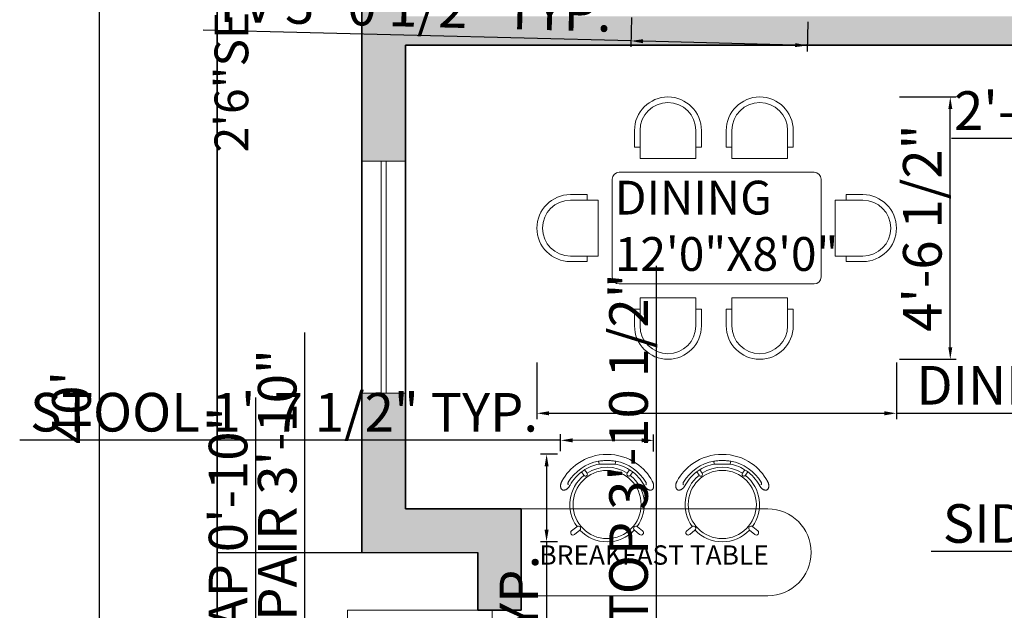
# Model space of a CAD drawing. Units: inches. Extents: x 4732 to 5926, y 2665 to 3255.
# Tile 3 of 8: x 4777 to 4982, y 2934 to 3056. Entities that reach past the tile are written whole.
import ezdxf

# ---------------------------------------------------------------- set-up
doc = ezdxf.new("R2010")
doc.units = ezdxf.units.IN
for name, color, linetype, lineweight in [('A-ANNO-DIMS', 2, 'Continuous', 18), ('A-ANNO-TEXT', 7, 'Continuous', 18), ('A-AREA-IDEN', 7, 'Continuous', 18), ('A-DOOR', 3, 'Continuous', 18), ('A-FLOR', 7, 'Continuous', 25), ('A-FLOR-CASE', 7, 'Continuous', 18), ('A-GLAZ', 4, 'Continuous', 18), ('A-WALL', 7, 'Continuous', 35), ('A-WALL-PATT', 8, 'Continuous', 13), ('C-PROP', 7, 'Continuous', 35), ('NOI THAT', 42, 'Continuous', 18)]:
    doc.layers.add(name, color=color, linetype=linetype, lineweight=lineweight)
doc.styles.get("Standard").update_dxf_attribs({"font": 'arial.ttf'})
doc.dimstyles.new('ISO-25', dxfattribs={"dimtxt": 8, "dimasz": 2.5, "dimexe": 1.25, "dimexo": 0.625, "dimtad": 1, "dimdec": 1, "dimlunit": 3, "dimtxsty": 'Standard', "dimcen": 2.5, "dimadec": 0, "dimazin": 0, "dimtfac": 1, "dimtdec": 1, "dimtmove": 0, "dimatfit": 3, "dimfxl": 1, "dimarcsym": 0})

# ---------------------------------------------------------------- blocks, each defined once
blk = doc.blocks.new('A$C3F0C2877')
at = {"layer": 'NOI THAT'}
for p, q in [((700, 1640), (700, 1520)), ((740, 1640), (740, 1440)), ((1140, 1440), (1140, 1640)), ((1180, 1520), (1180, 1640)), ((1358.3, 1640), (1358.3, 1520)), ((1398.3, 1640), (1398.3, 1440)), ((1798.3, 1440), (1798.3, 1640)), ((1838.3, 1520), (1838.3, 1640)), ((700, 1520), (740, 1520)), ((1140, 1520), (1180, 1520)), ((1358.3, 1520), (1398.3, 1520)), ((1798.3, 1520), (1838.3, 1520)), ((740, 1440), (1140, 1440)), ((1398.3, 1440), (1798.3, 1440)), ((540, 1290), (540, 590)), ((1988.3, 1340), (590, 1340)), ((2038.3, 590), (2038.3, 1290)), ((240, 1180), (360, 1180)), ((240, 1140), (440, 1140)), ((360, 1180), (360, 1140)), ((440, 1140), (440, 740)), ((2138.6, 1140), (2138.6, 740)), ((2338.6, 1140), (2138.6, 1140)), ((2338.6, 1180), (2218.6, 1180)), ((2218.6, 1180), (2218.6, 1140)), ((440, 740), (240, 740)), ((360, 740), (360, 700)), ((2138.6, 740), (2338.6, 740)), ((2218.6, 740), (2218.6, 700)), ((360, 700), (240, 700)), ((2218.6, 700), (2338.6, 700)), ((590, 540), (1988.3, 540)), ((740, 440), (1140, 440)), ((740, 240), (740, 440)), ((1140, 440), (1140, 240)), ((1398.3, 440), (1798.3, 440)), ((1398.3, 240), (1398.3, 440)), ((1798.3, 440), (1798.3, 240)), ((700, 360), (740, 360)), ((700, 240), (700, 360)), ((1140, 360), (1180, 360)), ((1180, 360), (1180, 240)), ((1358.3, 360), (1398.3, 360)), ((1358.3, 240), (1358.3, 360)), ((1798.3, 360), (1838.3, 360)), ((1838.3, 360), (1838.3, 240))]:
    blk.add_line(p, q, dxfattribs=at)
for centre, radius, start, end in [((940, 1640), 240, 0, 180), ((940, 1640), 200, 0, 180), ((1598.3, 1640), 240, 0, 180), ((1598.3, 1640), 200, 0, 180), ((590, 1290), 50, 90, 180), ((1988.3, 1290), 50, 0, 90), ((240, 940), 240, 90, 270), ((240, 940), 200, 90, 270), ((2338.6, 940), 240, 270, 90), ((2338.6, 940), 200, 270, 90), ((590, 590), 50, 180, 270), ((1988.3, 590), 50, 270, 0), ((940, 240), 240, 180, 0), ((940, 240), 200, 180, 0), ((1598.3, 240), 240, 180, 0), ((1598.3, 240), 200, 180, 0)]:
    blk.add_arc(centre, radius, start, end, dxfattribs=at)
blk = doc.blocks.new('SILLA 01')
for p, q in [((-0.1746, 0.2017), (-0.1626, 0.2119)), ((-0.1626, 0.2119), (-0.1501, 0.2213)), ((-0.1501, 0.2213), (-0.137, 0.23)), ((-0.137, 0.23), (-0.1234, 0.2379)), ((-0.1234, 0.2379), (-0.1216, 0.2388)), ((-0.1216, 0.2388), (-0.1198, 0.2397)), ((-0.1198, 0.2397), (-0.118, 0.2405)), ((-0.118, 0.2405), (-0.1161, 0.2412)), ((-0.1161, 0.2412), (-0.1143, 0.2419)), ((-0.1143, 0.2419), (-0.1124, 0.2426)), ((-0.1124, 0.2426), (-0.1104, 0.2431)), ((-0.1104, 0.2431), (-0.1085, 0.2437)), ((-0.1085, 0.2437), (-0.1069, 0.244)), ((-0.1069, 0.244), (-0.1053, 0.2444)), ((-0.1053, 0.2444), (-0.1037, 0.2446)), ((-0.1037, 0.2446), (-0.102, 0.2448)), ((-0.102, 0.2448), (-0.1004, 0.2449)), ((-0.1004, 0.2449), (-0.0987, 0.245)), ((-0.0987, 0.245), (-0.0971, 0.245)), ((-0.0971, 0.245), (-0.0954, 0.2449)), ((-0.0954, 0.2449), (-0.0939, 0.2448)), ((-0.0939, 0.2448), (-0.0924, 0.2446)), ((-0.0924, 0.2446), (-0.0908, 0.2443)), ((-0.0908, 0.2443), (-0.0893, 0.2439)), ((-0.0893, 0.2439), (-0.0878, 0.2435)), ((-0.0878, 0.2435), (-0.0864, 0.243)), ((-0.0864, 0.243), (-0.0849, 0.2423)), ((-0.0846, 0.208), (-0.0857, 0.2068)), ((-0.0849, 0.2423), (-0.0836, 0.2417)), ((-0.0835, 0.2093), (-0.0846, 0.208)), ((-0.0836, 0.2417), (-0.0826, 0.2411)), ((-0.0825, 0.2106), (-0.0835, 0.2093)), ((-0.0826, 0.2411), (-0.0817, 0.2405)), ((-0.0815, 0.212), (-0.0825, 0.2106)), ((-0.0817, 0.2405), (-0.0808, 0.2398)), ((-0.0806, 0.2133), (-0.0815, 0.212)), ((-0.0808, 0.2398), (-0.08, 0.239)), ((-0.0797, 0.2148), (-0.0806, 0.2133)), ((-0.08, 0.239), (-0.0792, 0.2382)), ((-0.0789, 0.2161), (-0.0797, 0.2148)), ((-0.0792, 0.2382), (-0.0785, 0.2373)), ((-0.0782, 0.2176), (-0.0789, 0.2161)), ((-0.0785, 0.2373), (-0.0779, 0.2364)), ((-0.0776, 0.219), (-0.0782, 0.2176)), ((-0.0779, 0.2364), (-0.0773, 0.2354)), ((-0.0771, 0.2205), (-0.0776, 0.219)), ((-0.0773, 0.2354), (-0.0769, 0.2344)), ((-0.0766, 0.222), (-0.0771, 0.2205)), ((-0.0769, 0.2344), (-0.0764, 0.2333)), ((-0.0762, 0.2235), (-0.0766, 0.222)), ((-0.0764, 0.2333), (-0.0761, 0.2322)), ((-0.0759, 0.2251), (-0.0762, 0.2235)), ((-0.0761, 0.2322), (-0.0759, 0.2311)), ((-0.0759, 0.2311), (-0.0757, 0.23)), ((-0.0757, 0.2266), (-0.0759, 0.2251)), ((-0.0757, 0.23), (-0.0756, 0.2289)), ((-0.0756, 0.2278), (-0.0757, 0.2266)), ((-0.0756, 0.2289), (-0.0756, 0.2278)), ((-0.2162, 0.1544), (-0.2068, 0.1672)), ((-0.2068, 0.1672), (-0.1968, 0.1793)), ((-0.1968, 0.1793), (-0.186, 0.1909)), ((-0.1896, 0.1368), (-0.1744, 0.1565)), ((-0.186, 0.1909), (-0.1746, 0.2017)), ((-0.1744, 0.1565), (-0.1571, 0.1744)), ((-0.1614, 0.1472), (-0.1525, 0.1566)), ((-0.1571, 0.1744), (-0.1381, 0.1904)), ((-0.1525, 0.1566), (-0.1432, 0.1655)), ((-0.1432, 0.1655), (-0.1334, 0.1739)), ((-0.1381, 0.1904), (-0.1176, 0.2043)), ((-0.1334, 0.1739), (-0.123, 0.1816)), ((-0.123, 0.1816), (-0.1123, 0.1887)), ((-0.1176, 0.2043), (-0.1159, 0.2052)), ((-0.1159, 0.2052), (-0.1142, 0.2058)), ((-0.1142, 0.2058), (-0.1123, 0.2062)), ((-0.1123, 0.2062), (-0.1104, 0.2063)), ((-0.1123, 0.1887), (-0.1012, 0.1952)), ((-0.1104, 0.2063), (-0.1086, 0.2062)), ((-0.1086, 0.2062), (-0.1067, 0.2058)), ((-0.1067, 0.2058), (-0.105, 0.2051)), ((-0.105, 0.2051), (-0.1033, 0.2042)), ((-0.0994, 0.1962), (-0.1012, 0.1952)), ((-0.0977, 0.1972), (-0.0994, 0.1962)), ((-0.096, 0.1983), (-0.0977, 0.1972)), ((-0.0943, 0.1994), (-0.096, 0.1983)), ((-0.0927, 0.2006), (-0.0943, 0.1994)), ((-0.0911, 0.2019), (-0.0927, 0.2006)), ((-0.0896, 0.2031), (-0.0911, 0.2019)), ((-0.0881, 0.2045), (-0.0896, 0.2031)), ((-0.0869, 0.2056), (-0.0881, 0.2045)), ((-0.0857, 0.2068), (-0.0869, 0.2056)), ((0.1136, 0.1509), (0.1141, 0.1558)), ((0.1141, 0.1558), (0.1165, 0.1601)), ((0.1165, 0.1601), (0.1387, 0.1871)), ((0.1577, 0.1709), (0.1354, 0.1439)), ((0.1387, 0.1871), (0.1425, 0.1901)), ((0.1425, 0.1901), (0.1471, 0.1915)), ((0.1471, 0.1915), (0.1519, 0.191)), ((0.1519, 0.191), (0.1561, 0.1886)), ((0.1561, 0.1886), (0.1592, 0.1848)), ((0.16, 0.1752), (0.1577, 0.1709)), ((0.1592, 0.1848), (0.1605, 0.1801)), ((0.1605, 0.1801), (0.16, 0.1752)), ((-0.245, 0.1003), (-0.2367, 0.1191)), ((-0.2367, 0.1191), (-0.2271, 0.1372)), ((-0.2271, 0.1372), (-0.2162, 0.1544)), ((-0.2136, 0.0931), (-0.2028, 0.1156)), ((-0.2028, 0.1156), (-0.1896, 0.1368)), ((-0.1945, 0.0969), (-0.1893, 0.1071)), ((-0.1893, 0.1071), (-0.1835, 0.1171)), ((-0.1835, 0.1171), (-0.1773, 0.1267)), ((-0.1828, 0.1184), (-0.1651, 0.1058)), ((-0.1773, 0.1267), (-0.1696, 0.1372)), ((-0.1538, 0.1223), (-0.1714, 0.1348)), ((-0.1696, 0.1372), (-0.1614, 0.1472)), ((-0.1616, 0.1042), (-0.1651, 0.1058)), ((-0.1577, 0.1041), (-0.1616, 0.1042)), ((-0.1541, 0.1055), (-0.1577, 0.1041)), ((-0.1513, 0.1083), (-0.1541, 0.1055)), ((-0.1538, 0.1223), (-0.1511, 0.1194)), ((-0.1498, 0.1118), (-0.1513, 0.1083)), ((-0.1511, 0.1194), (-0.1497, 0.1158)), ((-0.1497, 0.1158), (-0.1498, 0.1118)), ((0.115, 0.1462), (0.1136, 0.1509)), ((0.118, 0.1423), (0.115, 0.1462)), ((0.1222, 0.14), (0.118, 0.1423)), ((0.127, 0.1394), (0.1222, 0.14)), ((0.1317, 0.1408), (0.127, 0.1394)), ((0.1354, 0.1439), (0.1317, 0.1408)), ((-0.2609, 0.041), (-0.2571, 0.0611)), ((-0.2571, 0.0611), (-0.2518, 0.081)), ((-0.2518, 0.081), (-0.245, 0.1003)), ((-0.2281, 0.0453), (-0.2221, 0.0696)), ((-0.2221, 0.0696), (-0.2136, 0.0931)), ((-0.2125, 0.0422), (-0.2101, 0.0535)), ((-0.2101, 0.0535), (-0.207, 0.0646)), ((-0.207, 0.0646), (-0.2034, 0.0756)), ((-0.2034, 0.0756), (-0.1993, 0.0864)), ((-0.1993, 0.0864), (-0.1945, 0.0969)), ((-0.264, 0), (-0.2632, 0.0205)), ((-0.2632, -0.0205), (-0.264, 0)), ((-0.2632, 0.0205), (-0.2609, 0.041)), ((-0.2318, 0), (-0.2317, 0.0057)), ((-0.2317, -0.0057), (-0.2318, 0)), ((-0.2317, 0.0057), (-0.2315, 0.0114)), ((-0.2315, 0.0114), (-0.2312, 0.017)), ((-0.2312, 0.017), (-0.2307, 0.0227)), ((-0.2307, 0.0227), (-0.2301, 0.0283)), ((-0.2301, 0.0283), (-0.2294, 0.034)), ((-0.2294, 0.034), (-0.2285, 0.0396)), ((-0.2285, 0.0396), (-0.2275, 0.0452)), ((-0.2125, 0.0422), (-0.2275, 0.0452)), ((-0.2125, 0.0422), (-0.2125, -0.0422)), ((-0.2609, -0.041), (-0.2632, -0.0205)), ((-0.2571, -0.0611), (-0.2609, -0.041)), ((-0.2315, -0.0114), (-0.2317, -0.0057)), ((-0.2312, -0.017), (-0.2315, -0.0114)), ((-0.2307, -0.0227), (-0.2312, -0.017)), ((-0.2301, -0.0283), (-0.2307, -0.0227)), ((-0.2294, -0.034), (-0.2301, -0.0283)), ((-0.2285, -0.0396), (-0.2294, -0.034)), ((-0.2275, -0.0452), (-0.2285, -0.0396)), ((-0.2221, -0.0696), (-0.2281, -0.0453)), ((-0.2125, -0.0422), (-0.2275, -0.0452)), ((-0.2101, -0.0535), (-0.2125, -0.0422)), ((-0.2518, -0.081), (-0.2571, -0.0611)), ((-0.245, -0.1003), (-0.2518, -0.081)), ((-0.2367, -0.1191), (-0.245, -0.1003)), ((-0.2136, -0.0931), (-0.2221, -0.0696)), ((-0.2028, -0.1156), (-0.2136, -0.0931)), ((-0.207, -0.0646), (-0.2101, -0.0535)), ((-0.2034, -0.0756), (-0.207, -0.0646)), ((-0.1993, -0.0864), (-0.2034, -0.0756)), ((-0.1945, -0.0969), (-0.1993, -0.0864)), ((-0.1893, -0.1071), (-0.1945, -0.0969)), ((-0.2271, -0.1372), (-0.2367, -0.1191)), ((-0.2162, -0.1544), (-0.2271, -0.1372)), ((-0.2068, -0.1672), (-0.2162, -0.1544)), ((-0.1896, -0.1368), (-0.2028, -0.1156)), ((-0.1744, -0.1565), (-0.1896, -0.1368)), ((-0.1835, -0.1171), (-0.1893, -0.1071)), ((-0.1773, -0.1267), (-0.1835, -0.1171)), ((-0.1828, -0.1184), (-0.1651, -0.1058)), ((-0.1696, -0.1372), (-0.1773, -0.1267)), ((-0.1538, -0.1223), (-0.1714, -0.1348)), ((-0.1614, -0.1472), (-0.1696, -0.1372)), ((-0.1651, -0.1058), (-0.1616, -0.1042)), ((-0.1616, -0.1042), (-0.1577, -0.1041)), ((-0.1525, -0.1566), (-0.1614, -0.1472)), ((-0.1577, -0.1041), (-0.1541, -0.1055)), ((-0.1541, -0.1055), (-0.1513, -0.1083)), ((-0.1511, -0.1194), (-0.1538, -0.1223)), ((-0.1513, -0.1083), (-0.1498, -0.1118)), ((-0.1497, -0.1158), (-0.1511, -0.1194)), ((-0.1498, -0.1118), (-0.1497, -0.1158)), ((0.1136, -0.1509), (0.115, -0.1462)), ((0.1141, -0.1558), (0.1136, -0.1509)), ((0.115, -0.1462), (0.118, -0.1423)), ((0.118, -0.1423), (0.1222, -0.14)), ((0.1222, -0.14), (0.127, -0.1394)), ((0.127, -0.1394), (0.1317, -0.1408)), ((0.1317, -0.1408), (0.1354, -0.1439)), ((0.1577, -0.1709), (0.1354, -0.1439)), ((-0.1968, -0.1793), (-0.2068, -0.1672)), ((-0.186, -0.1909), (-0.1968, -0.1793)), ((-0.1746, -0.2017), (-0.186, -0.1909)), ((-0.1626, -0.2119), (-0.1746, -0.2017)), ((-0.1571, -0.1744), (-0.1744, -0.1565)), ((-0.1381, -0.1904), (-0.1571, -0.1744)), ((-0.1432, -0.1655), (-0.1525, -0.1566)), ((-0.1334, -0.1739), (-0.1432, -0.1655)), ((-0.1176, -0.2043), (-0.1381, -0.1904)), ((-0.123, -0.1816), (-0.1334, -0.1739)), ((-0.1123, -0.1887), (-0.123, -0.1816)), ((-0.1159, -0.2052), (-0.1176, -0.2043)), ((-0.1142, -0.2058), (-0.1159, -0.2052)), ((-0.1123, -0.2062), (-0.1142, -0.2058)), ((-0.1012, -0.1952), (-0.1123, -0.1887)), ((-0.1104, -0.2063), (-0.1123, -0.2062)), ((-0.1086, -0.2062), (-0.1104, -0.2063)), ((-0.1067, -0.2058), (-0.1086, -0.2062)), ((-0.105, -0.2051), (-0.1067, -0.2058)), ((-0.1033, -0.2042), (-0.105, -0.2051)), ((-0.1012, -0.1952), (-0.0994, -0.1962)), ((-0.0994, -0.1962), (-0.0977, -0.1972)), ((-0.0977, -0.1972), (-0.096, -0.1983)), ((-0.096, -0.1983), (-0.0943, -0.1994)), ((-0.0943, -0.1994), (-0.0927, -0.2006)), ((-0.0927, -0.2006), (-0.0911, -0.2019)), ((-0.0911, -0.2019), (-0.0896, -0.2031)), ((-0.0896, -0.2031), (-0.0881, -0.2045)), ((-0.0881, -0.2045), (-0.0869, -0.2056)), ((-0.0869, -0.2056), (-0.0857, -0.2068)), ((-0.0857, -0.2068), (-0.0846, -0.208)), ((0.1165, -0.1601), (0.1141, -0.1558)), ((0.1165, -0.1601), (0.1387, -0.1871)), ((0.1425, -0.1901), (0.1387, -0.1871)), ((0.1471, -0.1915), (0.1425, -0.1901)), ((0.1519, -0.191), (0.1471, -0.1915)), ((0.1561, -0.1886), (0.1519, -0.191)), ((0.1592, -0.1848), (0.1561, -0.1886)), ((0.1577, -0.1709), (0.16, -0.1752)), ((0.1605, -0.1801), (0.1592, -0.1848)), ((0.16, -0.1752), (0.1605, -0.1801)), ((-0.1501, -0.2213), (-0.1626, -0.2119)), ((-0.137, -0.23), (-0.1501, -0.2213)), ((-0.1234, -0.2379), (-0.137, -0.23)), ((-0.1216, -0.2388), (-0.1234, -0.2379)), ((-0.1198, -0.2397), (-0.1216, -0.2388)), ((-0.118, -0.2405), (-0.1198, -0.2397)), ((-0.1161, -0.2412), (-0.118, -0.2405)), ((-0.1143, -0.2419), (-0.1161, -0.2412)), ((-0.1124, -0.2426), (-0.1143, -0.2419)), ((-0.1104, -0.2431), (-0.1124, -0.2426)), ((-0.1085, -0.2437), (-0.1104, -0.2431)), ((-0.1069, -0.244), (-0.1085, -0.2437)), ((-0.1053, -0.2444), (-0.1069, -0.244)), ((-0.1037, -0.2446), (-0.1053, -0.2444)), ((-0.102, -0.2448), (-0.1037, -0.2446)), ((-0.1004, -0.2449), (-0.102, -0.2448)), ((-0.0987, -0.245), (-0.1004, -0.2449)), ((-0.0971, -0.245), (-0.0987, -0.245)), ((-0.0954, -0.2449), (-0.0971, -0.245)), ((-0.0939, -0.2448), (-0.0954, -0.2449)), ((-0.0924, -0.2446), (-0.0939, -0.2448)), ((-0.0908, -0.2443), (-0.0924, -0.2446)), ((-0.0893, -0.2439), (-0.0908, -0.2443)), ((-0.0878, -0.2435), (-0.0893, -0.2439)), ((-0.0864, -0.243), (-0.0878, -0.2435)), ((-0.0849, -0.2423), (-0.0864, -0.243)), ((-0.0836, -0.2417), (-0.0849, -0.2423)), ((-0.0846, -0.208), (-0.0835, -0.2093)), ((-0.0826, -0.2411), (-0.0836, -0.2417)), ((-0.0835, -0.2093), (-0.0825, -0.2106)), ((-0.0817, -0.2405), (-0.0826, -0.2411)), ((-0.0825, -0.2106), (-0.0815, -0.212)), ((-0.0808, -0.2398), (-0.0817, -0.2405)), ((-0.0815, -0.212), (-0.0806, -0.2133)), ((-0.08, -0.239), (-0.0808, -0.2398)), ((-0.0806, -0.2133), (-0.0797, -0.2148)), ((-0.0792, -0.2382), (-0.08, -0.239)), ((-0.0797, -0.2148), (-0.0789, -0.2161)), ((-0.0785, -0.2373), (-0.0792, -0.2382)), ((-0.0789, -0.2161), (-0.0782, -0.2176)), ((-0.0779, -0.2364), (-0.0785, -0.2373)), ((-0.0782, -0.2176), (-0.0776, -0.219)), ((-0.0773, -0.2354), (-0.0779, -0.2364)), ((-0.0776, -0.219), (-0.0771, -0.2205)), ((-0.0769, -0.2344), (-0.0773, -0.2354)), ((-0.0771, -0.2205), (-0.0766, -0.222)), ((-0.0764, -0.2333), (-0.0769, -0.2344)), ((-0.0766, -0.222), (-0.0762, -0.2235)), ((-0.0761, -0.2322), (-0.0764, -0.2333)), ((-0.0762, -0.2235), (-0.0759, -0.2251)), ((-0.0759, -0.2311), (-0.0761, -0.2322)), ((-0.0759, -0.2251), (-0.0757, -0.2266)), ((-0.0757, -0.23), (-0.0759, -0.2311)), ((-0.0757, -0.2266), (-0.0756, -0.2278)), ((-0.0756, -0.2289), (-0.0757, -0.23)), ((-0.0756, -0.2278), (-0.0756, -0.2289))]:
    blk.add_line(p, q)
blk.add_circle((0, 0), 0.1793)
for start, end in [(53.8818, 141.5278), (147.3489, 212.6511), (313.1989, 46.8011), (218.4722, 306.1182)]:
    blk.add_arc((0, 0), 0.196, start, end)
blk = doc.blocks.new('*U19')
for p, q in [((0, 0), (0, -6)), ((30, 0), (30, -6))]:
    blk.add_line(p, q)
blk.add_lwpolyline([(0, 0), (0, 30), (1.75, 30), (1.75, 0)], close=True)
blk.add_arc((0, 0), 30, 0, 90)
blk = doc.blocks.new('*D28')
at = {"layer": 'A-ANNO-DIMS', "color": 0, "lineweight": -2, "transparency": 16777216}
for p, q in [((4817.76, 3215.93), (4792.67, 3215.93)), ((4793.92, 3213.43), (4793.92, 2738.43)), ((4817.76, 2735.93), (4792.67, 2735.93))]:
    blk.add_line(p, q, dxfattribs=at)
at = {"layer": 'A-ANNO-DIMS', "color": 0, "transparency": 16777216}
for points in [[(4793.5, 3213.43), (4794.33, 3213.43), (4793.92, 3215.93)], [(4793.5, 2738.43), (4794.33, 2738.43), (4793.92, 2735.93)]]:
    blk.add_solid(points, dxfattribs=at)
at = {"layer": 'Defpoints', "color": 0, "transparency": 16777216}
for p in [(4818.38, 3215.93), (4793.92, 2735.93), (4818.38, 2735.93)]:
    blk.add_point(p, dxfattribs=at)
at = {"layer": 'A-ANNO-DIMS', "color": 0, "transparency": 16777216, "insert": (4789.21, 2975.93), "char_height": 8, "attachment_point": 5, "rotation": 90}
blk.add_mtext("40'", dxfattribs=at)
blk = doc.blocks.new('GLAZ-UNIT-48IN')
for p, q in [((0, 1), (48, 1)), ((0, 0), (48, 0))]:
    blk.add_line(p, q)
blk = doc.blocks.new('COUNTER-BREAKFAST')
for p, q in [((0, 18), (51.1, 18)), ((0, 0), (51.1, 0))]:
    blk.add_line(p, q)
blk.add_arc((51.1, 9), 9, 270, 90)
blk = doc.blocks.new('*D76')
at = {"layer": 'A-ANNO-DIMS', "color": 0, "lineweight": -2, "transparency": 16777216}
for p, q in [((4889.55, 2966.86), (4889.55, 2970.38)), ((4908.85, 2966.85), (4908.85, 2970.37)), ((4889.55, 2969.13), (4777.45, 2969.16)), ((4906.35, 2969.12), (4892.05, 2969.13))]:
    blk.add_line(p, q, dxfattribs=at)
at = {"layer": 'A-ANNO-DIMS', "color": 0, "transparency": 16777216}
for points in [[(4892.05, 2969.54), (4892.05, 2968.71), (4889.55, 2969.13)], [(4906.35, 2969.54), (4906.35, 2968.71), (4908.85, 2969.12)]]:
    blk.add_solid(points, dxfattribs=at)
at = {"layer": 'Defpoints', "color": 0, "transparency": 16777216}
for p in [(4889.55, 2969.13), (4889.55, 2966.23), (4908.85, 2966.23)]:
    blk.add_point(p, dxfattribs=at)
at = {"layer": 'A-ANNO-DIMS', "color": 0, "transparency": 16777216, "insert": (4832.25, 2973.91), "char_height": 8, "attachment_point": 5, "rotation": 359.9851}
blk.add_mtext('STOOL 1\'-7 1/2" TYP.', dxfattribs=at)
blk = doc.blocks.new('*D77')
at = {"layer": 'A-ANNO-DIMS', "color": 0, "lineweight": -2, "transparency": 16777216}
for p, q in [((4888.93, 2966.23), (4885.41, 2966.23)), ((4886.66, 2963.73), (4886.66, 2950.62)), ((4888.92, 2948.12), (4885.4, 2948.12)), ((4886.65, 2948.12), (4886.64, 2896.36))]:
    blk.add_line(p, q, dxfattribs=at)
at = {"layer": 'A-ANNO-DIMS', "color": 0, "transparency": 16777216}
for points in [[(4886.24, 2963.73), (4887.08, 2963.73), (4886.66, 2966.23)], [(4886.24, 2950.62), (4887.07, 2950.62), (4886.65, 2948.12)]]:
    blk.add_solid(points, dxfattribs=at)
at = {"layer": 'Defpoints', "color": 0, "transparency": 16777216}
for p in [(4889.55, 2966.23), (4886.65, 2948.12), (4889.55, 2948.12)]:
    blk.add_point(p, dxfattribs=at)
at = {"layer": 'A-ANNO-DIMS', "color": 0, "transparency": 16777216, "insert": (4881.94, 2920.99), "char_height": 8, "attachment_point": 5, "rotation": 89.9851}
blk.add_mtext('1\'-6" TYP.', dxfattribs=at)
blk = doc.blocks.new('*D79')
at = {"layer": 'A-ANNO-DIMS', "color": 0, "lineweight": -2, "transparency": 16777216}
for p, q in [((5041.84, 3027.77), (5041.84, 3032.86)), ((5066.25, 3027.77), (5066.25, 3032.86)), ((5041.84, 3031.61), (4970.55, 3031.61)), ((5063.75, 3031.61), (5044.34, 3031.61))]:
    blk.add_line(p, q, dxfattribs=at)
at = {"layer": 'A-ANNO-DIMS', "color": 0, "transparency": 16777216}
for points in [[(5044.34, 3032.03), (5044.34, 3031.2), (5041.84, 3031.61)], [(5063.75, 3032.03), (5063.75, 3031.2), (5066.25, 3031.61)]]:
    blk.add_solid(points, dxfattribs=at)
at = {"layer": 'Defpoints', "color": 0, "transparency": 16777216}
for p in [(5041.84, 3031.61), (5041.84, 3027.15), (5066.25, 3027.15)]:
    blk.add_point(p, dxfattribs=at)
at = {"layer": 'A-ANNO-DIMS', "color": 0, "transparency": 16777216, "insert": (5004.95, 3036.38), "char_height": 8, "attachment_point": 5}
blk.add_mtext('2\'-0 1/2" TYP.', dxfattribs=at)
blk = doc.blocks.new('*D82')
at = {"layer": 'A-ANNO-DIMS', "color": 0, "lineweight": -2, "transparency": 16777216}
for p, q in [((4904.29, 3056.7), (4904.13, 3050.59)), ((4940.81, 3055.77), (4940.65, 3049.66)), ((4904.16, 3051.84), (4815.45, 3054.1)), ((4938.19, 3050.98), (4906.66, 3051.78))]:
    blk.add_line(p, q, dxfattribs=at)
at = {"layer": 'A-ANNO-DIMS', "color": 0, "transparency": 16777216}
for points in [[(4906.67, 3052.2), (4906.65, 3051.36), (4904.16, 3051.84)], [(4938.2, 3051.39), (4938.17, 3050.56), (4940.68, 3050.91)]]:
    blk.add_solid(points, dxfattribs=at)
at = {"layer": 'Defpoints', "color": 0, "transparency": 16777216}
for p in [(4904.3, 3057.32), (4940.82, 3056.39), (4904.16, 3051.84)]:
    blk.add_point(p, dxfattribs=at)
at = {"layer": 'A-ANNO-DIMS', "color": 0, "transparency": 16777216, "insert": (4858.68, 3057.76), "char_height": 8, "attachment_point": 5, "rotation": 358.5431}
blk.add_mtext('TV 3\'-0 1/2" TYP.', dxfattribs=at)
blk = doc.blocks.new('*D86')
at = {"layer": 'A-ANNO-DIMS', "color": 0, "lineweight": -2, "transparency": 16777216}
for p, q in [((4836.57, 2874.85), (4836.57, 2991.43)), ((4842.86, 2874.85), (4835.32, 2874.85)), ((4836.57, 2831.25), (4836.57, 2872.35)), ((4842.86, 2828.75), (4835.32, 2828.75))]:
    blk.add_line(p, q, dxfattribs=at)
at = {"layer": 'A-ANNO-DIMS', "color": 0, "transparency": 16777216}
for points in [[(4836.16, 2872.35), (4836.99, 2872.35), (4836.57, 2874.85)], [(4836.16, 2831.25), (4836.99, 2831.25), (4836.57, 2828.75)]]:
    blk.add_solid(points, dxfattribs=at)
at = {"layer": 'Defpoints', "color": 0, "transparency": 16777216}
for p in [(4836.57, 2874.85), (4843.49, 2874.85), (4843.49, 2828.75)]:
    blk.add_point(p, dxfattribs=at)
at = {"layer": 'A-ANNO-DIMS', "color": 0, "transparency": 16777216, "insert": (4831.86, 2934.39), "char_height": 8, "attachment_point": 5, "rotation": 90}
blk.add_mtext('LAUNDRY PAIR 3\'-10"', dxfattribs=at)
blk = doc.blocks.new('*D88')
at = {"layer": 'A-ANNO-DIMS', "color": 0, "lineweight": -2, "transparency": 16777216}
for p, q in [((4884.65, 2985.28), (4884.65, 2973.48)), ((4959.16, 2985.28), (4959.16, 2973.48)), ((4887.15, 2974.73), (4956.66, 2974.73)), ((4959.16, 2974.73), (5069.48, 2974.73))]:
    blk.add_line(p, q, dxfattribs=at)
at = {"layer": 'A-ANNO-DIMS', "color": 0, "transparency": 16777216}
for points in [[(4887.15, 2975.15), (4887.15, 2974.31), (4884.65, 2974.73)], [(4956.66, 2975.15), (4956.66, 2974.31), (4959.16, 2974.73)]]:
    blk.add_solid(points, dxfattribs=at)
at = {"layer": 'Defpoints', "color": 0, "transparency": 16777216}
for p in [(4884.65, 2985.91), (4959.16, 2985.91), (4959.16, 2974.73)]:
    blk.add_point(p, dxfattribs=at)
at = {"layer": 'A-ANNO-DIMS', "color": 0, "transparency": 16777216, "insert": (5015.57, 2979.49), "char_height": 8, "attachment_point": 5}
blk.add_mtext('DINING SET 6\'-2 1/2"', dxfattribs=at)
blk = doc.blocks.new('*D89')
at = {"layer": 'A-ANNO-DIMS', "color": 0, "lineweight": -2, "transparency": 16777216}
for p, q in [((4959.78, 3040.23), (4971.58, 3040.23)), ((4970.33, 2988.41), (4970.33, 3037.73)), ((4959.78, 2985.91), (4971.58, 2985.91))]:
    blk.add_line(p, q, dxfattribs=at)
at = {"layer": 'A-ANNO-DIMS', "color": 0, "transparency": 16777216}
for points in [[(4969.92, 3037.73), (4970.75, 3037.73), (4970.33, 3040.23)], [(4969.92, 2988.41), (4970.75, 2988.41), (4970.33, 2985.91)]]:
    blk.add_solid(points, dxfattribs=at)
at = {"layer": 'Defpoints', "color": 0, "transparency": 16777216}
for p in [(4959.16, 3040.23), (4970.33, 3040.23), (4959.16, 2985.91)]:
    blk.add_point(p, dxfattribs=at)
at = {"layer": 'A-ANNO-DIMS', "color": 0, "transparency": 16777216, "insert": (4965.57, 3013.07), "char_height": 8, "attachment_point": 5, "rotation": 90}
blk.add_mtext('4\'-6 1/2"', dxfattribs=at)
blk = doc.blocks.new('*D90')
at = {"layer": 'A-ANNO-DIMS', "color": 0, "lineweight": -2, "transparency": 16777216}
for p, q in [((4909.45, 2896.49), (4909.45, 3005.26)), ((4903.1, 2896.49), (4910.7, 2896.49)), ((4909.45, 2852.54), (4909.45, 2893.99)), ((4903.1, 2850.04), (4910.7, 2850.04))]:
    blk.add_line(p, q, dxfattribs=at)
at = {"layer": 'A-ANNO-DIMS', "color": 0, "transparency": 16777216}
for points in [[(4909.03, 2893.99), (4909.86, 2893.99), (4909.45, 2896.49)], [(4909.03, 2852.54), (4909.86, 2852.54), (4909.45, 2850.04)]]:
    blk.add_solid(points, dxfattribs=at)
at = {"layer": 'Defpoints', "color": 0, "transparency": 16777216}
for p in [(4902.48, 2896.49), (4909.45, 2896.49), (4902.48, 2850.04)]:
    blk.add_point(p, dxfattribs=at)
at = {"layer": 'A-ANNO-DIMS', "color": 0, "transparency": 16777216, "insert": (4904.68, 2952.12), "char_height": 8, "attachment_point": 5, "rotation": 90}
blk.add_mtext('COOKTOP 3\'-10 1/2"', dxfattribs=at)
blk = doc.blocks.new('*D94')
at = {"layer": 'A-ANNO-DIMS', "color": 0, "lineweight": -2, "transparency": 16777216}
for p, q in [((5060.26, 2937.27), (5060.26, 2947.35)), ((5123.25, 2937.27), (5123.25, 2947.35)), ((5060.26, 2946.1), (4966.35, 2946.1)), ((5120.75, 2946.1), (5062.76, 2946.1))]:
    blk.add_line(p, q, dxfattribs=at)
at = {"layer": 'A-ANNO-DIMS', "color": 0, "transparency": 16777216}
for points in [[(5062.76, 2946.52), (5062.76, 2945.68), (5060.26, 2946.1)], [(5120.75, 2946.52), (5120.75, 2945.68), (5123.25, 2946.1)]]:
    blk.add_solid(points, dxfattribs=at)
at = {"layer": 'Defpoints', "color": 0, "transparency": 16777216}
for p in [(5060.26, 2946.1), (5060.26, 2936.65), (5123.25, 2936.65)]:
    blk.add_point(p, dxfattribs=at)
at = {"layer": 'A-ANNO-DIMS', "color": 0, "transparency": 16777216, "insert": (5012.05, 2950.87), "char_height": 8, "attachment_point": 5}
blk.add_mtext('SIDEBOARD 5\'-3"', dxfattribs=at)
blk = doc.blocks.new('*D102')
at = {"layer": 'A-ANNO-DIMS', "color": 0, "lineweight": -2, "transparency": 16777216}
for p, q in [((4826.38, 2877.6), (4826.38, 2977.97)), ((4825.51, 2877.6), (4827.63, 2877.6)), ((4826.38, 2870.1), (4826.38, 2875.1)), ((4825.51, 2867.6), (4827.63, 2867.6))]:
    blk.add_line(p, q, dxfattribs=at)
at = {"layer": 'A-ANNO-DIMS', "color": 0, "transparency": 16777216}
for points in [[(4825.96, 2875.1), (4826.8, 2875.1), (4826.38, 2877.6)], [(4825.96, 2870.1), (4826.8, 2870.1), (4826.38, 2867.6)]]:
    blk.add_solid(points, dxfattribs=at)
at = {"layer": 'Defpoints', "color": 0, "transparency": 16777216}
for p in [(4824.88, 2877.6), (4826.38, 2877.6), (4824.88, 2867.6)]:
    blk.add_point(p, dxfattribs=at)
at = {"layer": 'A-ANNO-DIMS', "color": 0, "transparency": 16777216, "insert": (4821.67, 2929.03), "char_height": 8, "attachment_point": 5, "rotation": 90}
blk.add_mtext('UTILITY TAP 0\'-10"', dxfattribs=at)

msp = doc.modelspace()

# ---------------------------------------------------------------- hatches: boundary and pattern name
at = {"layer": 'A-WALL-PATT'}
h = msp.add_hatch(color=256, dxfattribs=at)
h.dxf.hatch_style = 1
h.paths.add_polyline_path([(4905.38, 3185.93), (4848.38, 3185.93), (4848.38, 3146.93), (4857.38, 3146.93), (4857.38, 3176.93), (4905.38, 3176.93)])
h.paths.add_polyline_path([(5022.38, 3185.93), (4953.38, 3185.93), (4953.38, 3176.93), (4966.1, 3176.93), (5001.38, 3176.93), (5001.38, 3098.93), (5028.38, 3098.93), (5028.38, 3104.93), (5007.38, 3104.93), (5007.38, 3176.93), (5022.38, 3176.93)])
h.paths.add_polyline_path([(5115.38, 3185.93), (5046.38, 3185.93), (5046.38, 3176.93), (5061.38, 3176.93), (5061.38, 3104.93), (5058.38, 3104.93), (5058.38, 3098.93), (5067.38, 3098.93), (5067.38, 3176.93), (5115.38, 3176.93)])
h.paths.add_polyline_path([(5220.38, 3185.93), (5163.38, 3185.93), (5163.38, 3176.93), (5168.97, 3176.93), (5211.38, 3176.93), (5211.38, 3146.93), (5220.38, 3146.93)])
h.paths.add_polyline_path([(4857.38, 3086.93), (4848.38, 3086.93), (4848.38, 3026.93), (4857.38, 3026.93), (4857.38, 3050.93), (5001.38, 3050.93), (5001.38, 3008.93), (5007.38, 3008.93), (5007.38, 3050.93), (5022.38, 3050.93), (5022.38, 3056.93), (4857.38, 3056.93)])
h.paths.add_polyline_path([(4857.38, 2978.93), (4848.38, 2978.93), (4848.38, 2945.93), (4872.38, 2945.93), (4872.38, 2933.93), (4875.38, 2933.93), (4881.38, 2933.93), (4881.38, 2954.93), (4857.38, 2954.93)])
h.paths.add_polyline_path([(4881.38, 2903.93), (4875.38, 2903.93), (4872.38, 2903.93), (4872.38, 2897.93), (4881.38, 2897.93)])
h.paths.add_polyline_path([(4881.38, 2849.93), (4872.38, 2849.93), (4872.38, 2828.75), (4872.38, 2825.93), (4848.38, 2825.93), (4848.38, 2804.93), (4857.38, 2804.93), (4857.38, 2816.93), (4929.38, 2816.93), (4929.38, 2825.93), (4881.38, 2825.93)])
h.paths.add_polyline_path([(4975.38, 2744.93), (4857.38, 2744.93), (4857.38, 2756.93), (4848.38, 2756.93), (4848.38, 2735.93), (4975.38, 2735.93)])
h.paths.add_polyline_path([(5160.38, 2915.93), (5160.38, 2918.93), (5007.38, 2918.93), (5007.38, 2960.93), (5001.38, 2960.93), (5001.38, 2825.93), (4977.38, 2825.93), (4977.38, 2816.93), (5010.38, 2816.93), (5010.38, 2909.93), (5160.38, 2909.93)])
h.paths.add_polyline_path([(5220.38, 2948.93), (5211.38, 2948.93), (5211.38, 2918.93), (5208.38, 2918.93), (5208.38, 2909.93), (5220.38, 2909.93)])
h.paths.add_polyline_path([(5220.38, 3086.93), (5211.38, 3086.93), (5211.38, 3056.93), (5106.38, 3056.93), (5106.38, 3050.93), (5211.38, 3050.93), (5211.38, 3020.93), (5220.38, 3020.93)])
h.paths.add_polyline_path([(5067.38, 3098.93), (5061.38, 3098.93), (5061.38, 3056.93), (5058.38, 3056.93), (5058.38, 3050.93), (5061.38, 3050.93), (5070.38, 3050.93), (5070.38, 3056.93), (5067.38, 3056.93)])
h.paths.add_polyline_path([(4883.76, 2941.13), (4938.24, 2941.13), (4938.24, 2949.38), (4883.76, 2949.38)], flags=9)
h.paths.add_polyline_path([(4840.48, 3026.79), (4840.48, 3093.88), (4825.54, 3093.88), (4825.54, 3026.79)], flags=9)
h.paths.add_polyline_path([(5245.66, 2994.98), (5245.66, 3062.07), (5230.72, 3062.07), (5230.72, 2994.98)], flags=9)
h.paths.add_polyline_path([(4994.89, 3193.24), (5061.99, 3193.24), (5061.99, 3208.18), (4994.89, 3208.18)], flags=9)
h.paths.add_polyline_path([(5081.53, 3115.35), (5081.53, 3161.13), (5073.28, 3161.13), (5073.28, 3115.35)], flags=25)
h.paths.add_polyline_path([(4997.53, 3115.35), (4997.53, 3161.13), (4989.28, 3161.13), (4989.28, 3115.35)], flags=25)
h.paths.add_polyline_path([(5175.31, 2866.04), (5202.42, 2866.04), (5202.42, 2876.71), (5175.31, 2876.71)], flags=9)
h.paths.add_polyline_path([(4820.13, 2876.28), (4869.1, 2876.28), (4869.1, 2902.89), (4820.13, 2902.89)], flags=9)
h.paths.add_polyline_path([(5104.69, 2868.81), (5158.82, 2868.81), (5158.82, 2895.42), (5104.69, 2895.42)], flags=25)
h.paths.add_polyline_path([(5084.11, 2966.75), (5138.25, 2966.75), (5138.25, 2993.36), (5084.11, 2993.36)], flags=9)
h.paths.add_polyline_path([(4897.84, 3000.24), (4946.81, 3000.24), (4946.81, 3026.85), (4897.84, 3026.85)], flags=9)
h.paths.add_polyline_path([(5009.53, 3133.48), (5059.32, 3133.48), (5059.32, 3160.09), (5009.53, 3160.09)], flags=9)
h.paths.add_polyline_path([(5124.24, 3088.37), (5180.47, 3088.37), (5180.47, 3114.99), (5124.24, 3114.99)], flags=9)
h.paths.add_polyline_path([(4897.52, 3088.37), (4965.52, 3088.37), (4965.52, 3114.99), (4897.52, 3114.99)], flags=9)
h.paths.add_polyline_path([(4924.5, 2879.19), (4978.63, 2879.19), (4978.63, 2905.8), (4924.5, 2905.8)], flags=9)

# ---------------------------------------------------------------- linework, layer by layer
at = {"layer": 'A-FLOR'}
msp.add_line((4818.38, 2945.93), (4872.38, 2945.93), dxfattribs=at)
at = {"layer": 'A-GLAZ'}
for p, q in [((4857.38, 3026.93), (4848.38, 3026.93)), ((4857.38, 2978.93), (4848.38, 2978.93))]:
    msp.add_line(p, q, dxfattribs=at)
at = {"layer": 'A-WALL'}
for p, q in [((4848.38, 2945.93), (4848.38, 3185.93)), ((4857.38, 3050.93), (5001.38, 3050.93)), ((4857.38, 2954.93), (4857.38, 3050.93)), ((4857.38, 2954.93), (4881.38, 2954.93)), ((4881.38, 2933.93), (4881.38, 2954.93)), ((4872.38, 2933.93), (4872.38, 2945.93)), ((4872.38, 2933.93), (4881.38, 2933.93))]:
    msp.add_line(p, q, dxfattribs=at)
at = {"layer": 'C-PROP'}
msp.add_lwpolyline([(4818.38, 3215.93), (5250.38, 3215.93), (5250.38, 2735.93), (4818.38, 2735.93)], close=True, dxfattribs=at)

# ---------------------------------------------------------------- block references
at = {"layer": 'A-DOOR', "xscale": -1, "rotation": 90}
msp.add_blockref('*U19', (4875.38, 2933.93), dxfattribs=at)
at = {"layer": 'A-FLOR-CASE'}
msp.add_blockref('COUNTER-BREAKFAST', (4881.38, 2936.93), dxfattribs=at)
at = {"layer": 'A-GLAZ', "rotation": 269.9999999999978}
msp.add_blockref('GLAZ-UNIT-48IN', (4852.38, 3026.93), dxfattribs=at)
at = {"layer": 'NOI THAT', "xscale": 0.0288952394299788, "yscale": 0.0288952394299788, "zscale": 0.0288952394299788}
msp.add_blockref('A$C3F0C2877', (4884.65, 2985.91), dxfattribs=at)
at = {"layer": 'NOI THAT', "xscale": -39.375, "yscale": 39.375, "zscale": 39.375, "rotation": 89.9851020010651}
for p in [(4899.2, 2955.83), (4923.07, 2955.83)]:
    msp.add_blockref('SILLA 01', p, dxfattribs=at)

# ---------------------------------------------------------------- texts
at = {"layer": 'A-ANNO-TEXT', "insert": (4817.83, 3028.76), "char_height": 7, "attachment_point": 1, "rotation": 90}
msp.add_mtext_dynamic_manual_height_columns('{\\fTimes New Roman|b0|i0|c0|p18; 2\'6"SETBACK }', width=61.0557, gutter_width=12.5, heights=[0], dxfattribs=at)
at = {"layer": 'A-ANNO-TEXT', "insert": (4885.17, 2947.38), "char_height": 4, "attachment_point": 1}
msp.add_mtext_dynamic_manual_height_columns('BREAKFAST TABLE', width=72.2298, gutter_width=12.5, heights=[0], dxfattribs=at)
at = {"layer": 'A-AREA-IDEN', "insert": (4900.8, 3022.89), "char_height": 7, "attachment_point": 1}
msp.add_mtext_dynamic_manual_height_columns('{\\fTimes New Roman|b0|i0|c0|p18;DINING\\P12\'0"X8\'0"}', width=61.0557, gutter_width=12.5, heights=[0], dxfattribs=at)

# ---------------------------------------------------------------- dimensions: what is measured, and where the dimension line sits
at = {"layer": 'A-ANNO-DIMS'}
for base, p1, p2, override, picture, middle in [((4793.92, 2735.93), (4818.38, 3215.93), (4818.38, 2735.93), {"dimclrd": 0, "dimclre": 0, "dimclrt": 0}, '*D28', (4789.21, 2975.93)), ((4970.33, 3040.23), (4959.16, 2985.91), (4959.16, 3040.23), {"dimdec": 1, "dimlfac": 1, "dimrnd": 0, "dimzin": 1, "dimdsep": 46, "dimlunit": 4, "dimfrac": 2}, '*D89', (4965.57, 3013.07))]:
    dim = msp.add_linear_dim(base=base, p1=p1, p2=p2, angle=90, dimstyle='ISO-25', override=override, dxfattribs=at)
    dim.commit()
    dim.dimension.update_dxf_attribs({"geometry": picture, "text_midpoint": middle})
for base, p1, p2, angle, text, picture, middle in [((4904.16, 3051.84), (4940.82, 3056.39), (4904.3, 3057.32), 178.5431, 'TV <> TYP.', '*D82', (4858.68, 3057.76)), ((5041.84, 3031.61), (5066.25, 3027.15), (5041.84, 3027.15), 180, '<> TYP.', '*D79', (5004.95, 3036.38)), ((4909.4455, 2896.487), (4902.4785, 2850.0405), (4902.4785, 2896.487), 90, 'COOKTOP <>', '*D90', (4904.6786, 2952.1222)), ((4889.55, 2969.13), (4908.85, 2966.23), (4889.55, 2966.23), 179.9851, 'STOOL <> TYP.', '*D76', (4832.25, 2973.91)), ((4836.57, 2874.85), (4843.49, 2828.75), (4843.49, 2874.85), 90, 'LAUNDRY PAIR <>', '*D86', (4831.86, 2934.39)), ((4826.38, 2877.6), (4824.88, 2867.6), (4824.88, 2877.6), 90, 'UTILITY TAP <>', '*D102', (4821.67, 2929.03)), ((4886.65, 2948.12), (4889.55, 2966.23), (4889.55, 2948.12), 269.9851, '<> TYP.', '*D77', (4881.94, 2920.99)), ((5060.26, 2946.1), (5123.25, 2936.65), (5060.26, 2936.65), 180, 'SIDEBOARD <>', '*D94', (5012.05, 2950.87))]:
    dim = msp.add_linear_dim(base=base, p1=p1, p2=p2, angle=angle, text=text, dimstyle='ISO-25', override={"dimdec": 1, "dimlfac": 1, "dimrnd": 0, "dimzin": 1, "dimdsep": 46, "dimlunit": 4, "dimfrac": 2}, dxfattribs=at)
    dim.commit()
    dim.dimension.update_dxf_attribs({"geometry": picture, "text_midpoint": middle})
dim = msp.add_linear_dim(base=(4959.16, 2974.73), p1=(4884.65, 2985.91), p2=(4959.16, 2985.91), text='DINING SET <>', dimstyle='ISO-25', override={"dimdec": 1, "dimlfac": 1, "dimrnd": 0, "dimzin": 1, "dimdsep": 46, "dimlunit": 4, "dimfrac": 2}, dxfattribs=at)
dim.commit()
dim.dimension.update_dxf_attribs({"geometry": '*D88', "text_midpoint": (5015.57, 2979.49)})

doc.saveas('drawing.dxf')
